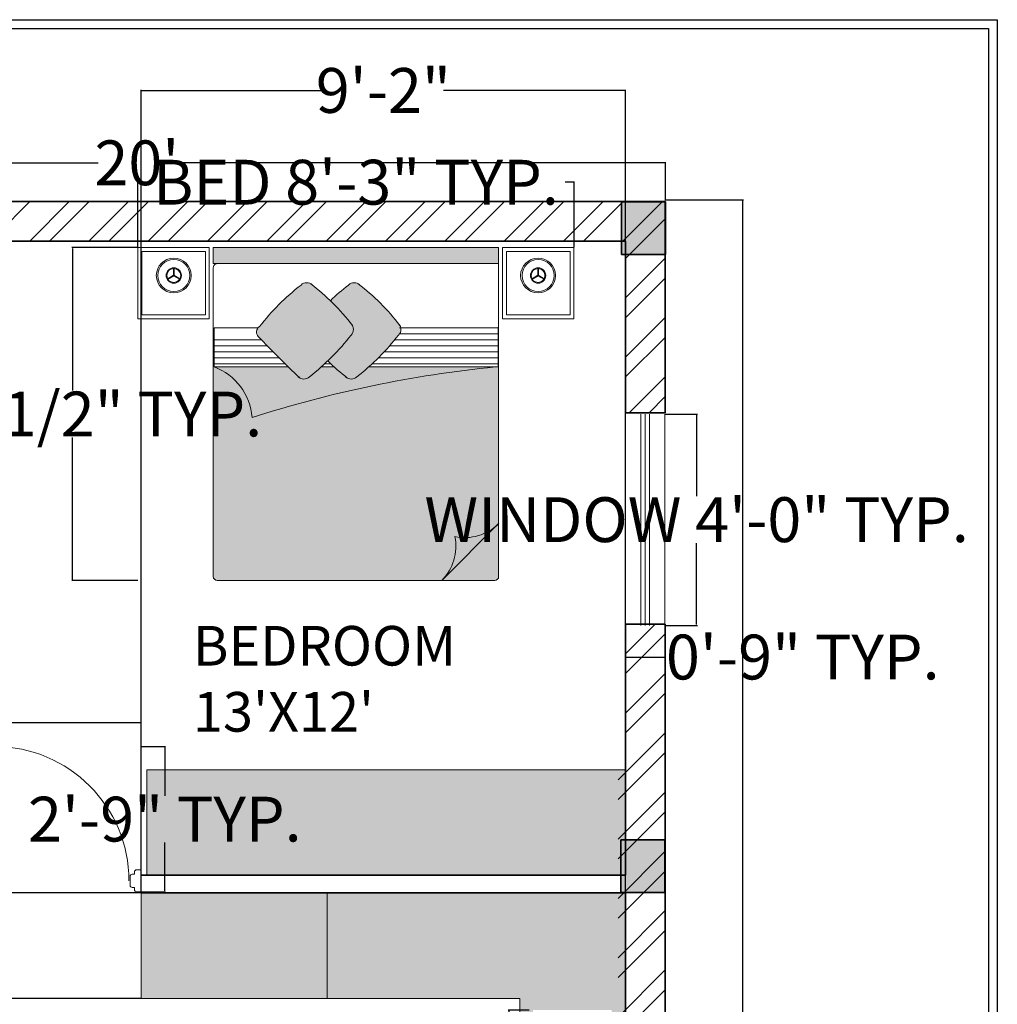
# Model space of a CAD drawing. Units: inches. Extents: x 1812 to 2791, y 2306 to 2959.
# Tile 4 of 8: x 1984 to 2206, y 2715 to 2939. Entities that reach past the tile are written whole.
import ezdxf

# ---------------------------------------------------------------- set-up
doc = ezdxf.new("R2010")
doc.units = ezdxf.units.IN
doc.layers.get('Defpoints').update_dxf_attribs({"lineweight": 50})
for name, color, linetype, lineweight in [('00 FURNITURE', 15, 'Continuous', 15), ('A-ANNO-DIMS', 2, 'Continuous', 18), ('A-ANNO-TTLB', 7, 'Continuous', 25), ('A-AREA-IDEN', 7, 'Continuous', 18), ('A-COLS', 7, 'Continuous', 35), ('A-FLOR-CASE', 8, 'Continuous', 18), ('A-WALL-PATT', 8, 'Continuous', 13), ('DOORS', 4, 'Continuous', 18), ('WALL', 7, 'Continuous', 35), ('WINDOWS', 160, 'Continuous', 18)]:
    doc.layers.add(name, color=color, linetype=linetype, lineweight=lineweight)
doc.layers.add('A-FURN-PATT', color=241, linetype='Continuous', lineweight=9, true_color=0xf7abae)
doc.styles.get("Standard").update_dxf_attribs({"font": 'arial.ttf'})
doc.dimstyles.get("Standard").update_dxf_attribs({"dimtxt": 10.18, "dimasz": 0.18, "dimexe": 0.18, "dimexo": 0.0625, "dimgap": 0.09, "dimtad": 0, "dimtih": 1, "dimtoh": 1, "dimdec": 0, "dimzin": 0, "dimdsep": 46, "dimlunit": 3, "dimtxsty": 'Standard', "dimcen": 0.09, "dimadec": 0, "dimazin": 0, "dimtfac": 1, "dimtdec": 0, "dimtofl": 0, "dimtmove": 0, "dimatfit": 3, "dimfxl": 1, "dimtolj": 1, "dimtzin": 0, "dimarcsym": 0})

# ---------------------------------------------------------------- blocks, each defined once
blk = doc.blocks.new('RGWTG')
at = {"layer": '00 FURNITURE'}
for p, q in [((578.23, 3473.51), (577.36, 3475.01)), ((578.23, 3473.58), (577.36, 3472.08)), ((578.36, 3473.58), (577.49, 3475.09)), ((578.36, 3473.51), (577.49, 3472)), ((578.29, 3473.62), (580.03, 3473.62)), ((578.29, 3473.47), (580.03, 3473.47)), ((521.93, 3464.58), (509.03, 3451.68)), ((509.93, 3464.58), (566.4, 3464.58)), ((557.53, 3463.84), (557.53, 3464.49)), ((557.53, 3464.49), (566.4, 3464.49)), ((558.2, 3464.49), (558.2, 3435.82)), ((559.57, 3464.49), (559.57, 3437.25)), ((560.94, 3464.49), (560.94, 3438.58)), ((562.3, 3464.49), (562.3, 3439.83)), ((563.67, 3464.49), (563.67, 3440.99)), ((565.04, 3464.49), (565.04, 3442.08)), ((566.4, 3464.58), (580.98, 3464.58)), ((566.4, 3464.49), (566.4, 3442.08)), ((566.4, 3464.49), (566.4, 3463.84)), ((580.98, 3464.58), (580.98, 3416.72)), ((509.03, 3422.63), (509.03, 3463.68)), ((558.2, 3426.48), (558.2, 3425.04)), ((509.03, 3400.68), (509.03, 3422.63)), ((558.2, 3416.13), (558.2, 3399.95)), ((580.98, 3416.72), (580.98, 3400.68)), ((559.57, 3414.75), (559.57, 3399.95)), ((560.94, 3413.39), (560.94, 3399.95)), ((562.3, 3412.04), (562.3, 3399.95)), ((563.67, 3410.72), (563.67, 3399.95)), ((580.08, 3399.78), (509.93, 3399.78)), ((557.53, 3399.95), (557.53, 3400.6)), ((566.4, 3399.95), (557.53, 3399.95)), ((566.4, 3400.6), (566.4, 3399.95)), ((578.23, 3390.78), (577.36, 3392.29)), ((578.23, 3390.86), (577.36, 3389.36)), ((578.36, 3390.86), (577.49, 3392.36)), ((578.36, 3390.78), (577.49, 3389.28)), ((578.29, 3390.9), (580.03, 3390.9)), ((578.29, 3390.74), (580.03, 3390.74))]:
    blk.add_line(p, q, dxfattribs=at)
for points in [[(568.43, 3465.48), (584.63, 3465.48), (584.63, 3481.68), (568.43, 3481.68)], [(569.33, 3466.38), (583.73, 3466.38), (583.73, 3480.78), (569.33, 3480.78)], [(580.98, 3399.78), (584.63, 3399.78), (584.63, 3464.58), (580.98, 3464.58)], [(568.43, 3398.88), (584.63, 3398.88), (584.63, 3382.68), (568.43, 3382.68)], [(569.33, 3397.98), (583.73, 3397.98), (583.73, 3383.58), (569.33, 3383.58)]]:
    blk.add_lwpolyline(points, close=True, dxfattribs=at)
for points in [[(566.52, 3464.49), (557.53, 3464.49), (557.53, 3435.08)], [(557.53, 3427.21), (557.53, 3424.3)], [(557.53, 3416.82), (557.53, 3399.95), (566.4, 3399.95), (566.4, 3409.94)]]:
    blk.add_lwpolyline(points, dxfattribs=at)
for centre, radius in [((578.29, 3473.54), 3.97), ((578.29, 3473.54), 3.63), ((578.29, 3473.54), 1.74), ((578.29, 3473.54), 1.56), ((578.29, 3390.82), 3.97), ((578.29, 3390.82), 3.63), ((578.29, 3390.82), 1.74), ((578.29, 3390.82), 1.56)]:
    blk.add_circle(centre, radius, dxfattribs=at)
for centre, radius, start, end in [((509.93, 3463.68), 0.9, 90, 180), ((529.65, 3456.88), 10.9, 135.0361, 191.9278), ((290.56, 3490.52), 268.3, 342.2214, 354.2925), ((516.73, 3443.97), 10.9, 78.0722, 134.9639), ((566.05, 3440.57), 1.82, 45, 135), ((533.58, 3399.31), 54.32, 37.931, 52.069), ((598.15, 3399.01), 54.32, 127.931, 142.069), ((574.84, 3431.77), 1.82, 315, 45), ((556.59, 3431.11), 1.82, 135, 225), ((598.15, 3388.23), 54.32, 127.931, 142.069), ((566.05, 3429.78), 1.82, 45, 135), ((533.58, 3388.53), 54.32, 37.931, 52.069), ((597.87, 3463.6), 54.32, 217.931, 224.141), ((533.28, 3463.88), 54.32, 316.32, 322.069), ((574.84, 3420.99), 1.82, 315, 45), ((556.59, 3420.33), 1.82, 135, 225), ((533.28, 3453.1), 54.32, 307.931, 322.069), ((765.33, 3619.75), 290.45, 223.6069, 226.2326), ((545.02, 3395.29), 13.35, 20.4224, 85.5825), ((565.44, 3411.05), 1.47, 225.9674, 326.8337), ((509.93, 3400.68), 0.9, 180, 270), ((580.08, 3400.68), 0.9, 270, 0)]:
    blk.add_arc(centre, radius, start, end, dxfattribs=at)
blk = doc.blocks.new('DDD')
at = {"layer": '00 FURNITURE'}
for p, q in [((-12579.77, -15859.53), (-12579.77, -15829.05)), ((-12578.77, -15859.53), (-12578.77, -15829.03)), ((-12612.02, -15857.03), (-12612.02, -15862.03)), ((-12611.02, -15857.03), (-12612.02, -15857.03)), ((-12610.52, -15858.03), (-12610.52, -15857.53)), ((-12577.52, -15858.03), (-12577.52, -15857.53)), ((-12577.02, -15857.03), (-12576.02, -15857.03)), ((-12576.02, -15857.03), (-12576.02, -15862.03)), ((-12578.77, -15859.53), (-12579.77, -15859.53)), ((-12612.02, -15862.03), (-12611.02, -15862.03)), ((-12610.52, -15861.53), (-12610.52, -15861.03)), ((-12577.52, -15861.53), (-12577.52, -15861.03)), ((-12576.02, -15862.03), (-12577.02, -15862.03))]:
    blk.add_line(p, q, dxfattribs=at)
for points in [[(-12610.52, -15861.03), (-12610.02, -15861.03, 0.414214), (-12609.52, -15860.53), (-12609.52, -15858.53, 0.414214), (-12610.02, -15858.03), (-12610.52, -15858.03)], [(-12577.52, -15861.03), (-12578.02, -15861.03, -0.414214), (-12578.52, -15860.53), (-12578.52, -15858.53, -0.414214), (-12578.02, -15858.03), (-12577.52, -15858.03)]]:
    blk.add_lwpolyline(points, format="xyb", dxfattribs=at)
for centre, radius, start, end in [((-12578.77, -15859.53), 30.5, 90, 180), ((-12611.02, -15857.53), 0.5, 0, 90), ((-12577.02, -15857.53), 0.5, 90, 180), ((-12611.02, -15861.53), 0.5, 270, 0), ((-12577.02, -15861.53), 0.5, 180, 270)]:
    blk.add_arc(centre, radius, start, end, dxfattribs=at)
blk = doc.blocks.new('*D14')
at = {"layer": 'A-ANNO-DIMS', "color": 0, "lineweight": -2, "transparency": 16777216}
for p, q in [((1890.37, 2897.89), (1890.37, 2906.59)), ((1890.55, 2906.41), (2001.61, 2906.41)), ((2130.3, 2906.41), (2019.24, 2906.41)), ((2130.48, 2897.89), (2130.48, 2906.59))]:
    blk.add_line(p, q, dxfattribs=at)
at = {"layer": 'A-ANNO-DIMS', "color": 0, "transparency": 16777216}
for points in [[(1890.55, 2906.44), (1890.55, 2906.38), (1890.37, 2906.41)], [(2130.3, 2906.44), (2130.3, 2906.38), (2130.48, 2906.41)]]:
    blk.add_solid(points, dxfattribs=at)
at = {"layer": 'Defpoints', "color": 0, "transparency": 16777216}
for p in [(2130.48, 2906.41), (1890.37, 2897.82), (2130.48, 2897.82)]:
    blk.add_point(p, dxfattribs=at)
at = {"layer": 'A-ANNO-DIMS', "color": 0, "transparency": 16777216, "insert": (2010.42, 2906.41), "char_height": 10.18, "attachment_point": 5}
blk.add_mtext("\\A1;20'", dxfattribs=at)
blk = doc.blocks.new('*D15')
at = {"layer": 'A-ANNO-DIMS', "color": 0, "lineweight": -2, "transparency": 16777216}
for p, q in [((2130.4, 2898), (2148.13, 2898)), ((2147.95, 2897.82), (2147.95, 2663.08)), ((2147.95, 2417.77), (2147.95, 2652.51)), ((2130.4, 2417.59), (2148.13, 2417.59))]:
    blk.add_line(p, q, dxfattribs=at)
at = {"layer": 'A-ANNO-DIMS', "color": 0, "transparency": 16777216}
for points in [[(2147.92, 2897.82), (2147.98, 2897.82), (2147.95, 2898)], [(2147.92, 2417.77), (2147.98, 2417.77), (2147.95, 2417.59)]]:
    blk.add_solid(points, dxfattribs=at)
at = {"layer": 'Defpoints', "color": 0, "transparency": 16777216}
for p in [(2130.34, 2898), (2130.34, 2417.59), (2147.95, 2417.59)]:
    blk.add_point(p, dxfattribs=at)
at = {"layer": 'A-ANNO-DIMS', "color": 0, "transparency": 16777216, "insert": (2147.95, 2657.8), "char_height": 10.18, "attachment_point": 5}
blk.add_mtext("\\A1;40'", dxfattribs=at)
blk = doc.blocks.new('COL')
at = {"transparency": 33554687}
h = blk.add_hatch(color=256, dxfattribs=at)
h.dxf.hatch_style = 1
h.paths.add_polyline_path([(2424.4, 2829.24), (2424.4, 2839.24), (2412.4, 2839.24), (2412.4, 2829.24)])
for p, q in [((2412.4, 2839.24), (2424.4, 2839.24)), ((2412.4, 2839.24), (2412.4, 2829.24)), ((2424.4, 2839.24), (2424.4, 2829.24)), ((2412.4, 2829.24), (2424.4, 2829.24))]:
    blk.add_line(p, q)
blk = doc.blocks.new('WINDOW-48x9')
for p, q in [((0, 48), (0, 0)), ((3.5, 0), (3.5, 48)), ((4.5, 0), (4.5, 48)), ((5.5, 0), (5.5, 48)), ((9, 0), (9, 48))]:
    blk.add_line(p, q)
blk = doc.blocks.new('SHEET-FRAME-RESIDENCE')
blk.add_lwpolyline([(0, 632.8), (378.76, 632.8), (378.76, 0), (0, 0)], close=True)
blk.add_lwpolyline([(2, 71.32), (2, 630.8), (376.76, 630.8), (376.76, 71.32)])
blk = doc.blocks.new('*D42')
at = {"layer": 'A-ANNO-DIMS', "color": 0, "lineweight": -2, "transparency": 16777216}
for p, q in [((1975.37, 2779.24), (1975.19, 2779.24)), ((1975.37, 2773.9), (1975.37, 2779.42)), ((2011.19, 2779.24), (1975.55, 2779.24)), ((2011.37, 2773.9), (2011.37, 2779.42))]:
    blk.add_line(p, q, dxfattribs=at)
at = {"layer": 'A-ANNO-DIMS', "color": 0, "transparency": 16777216}
for points in [[(1975.55, 2779.27), (1975.55, 2779.21), (1975.37, 2779.24)], [(2011.19, 2779.27), (2011.19, 2779.21), (2011.37, 2779.24)]]:
    blk.add_solid(points, dxfattribs=at)
at = {"layer": 'Defpoints', "color": 0, "transparency": 16777216}
for p in [(1975.37, 2779.24), (1975.37, 2773.84), (2011.37, 2773.84)]:
    blk.add_point(p, dxfattribs=at)
at = {"layer": 'A-ANNO-DIMS', "color": 0, "transparency": 16777216, "insert": (1921.02, 2779.24), "char_height": 10.18, "attachment_point": 5}
blk.add_mtext('\\A1;DOOR 3\'-0" TYP.', dxfattribs=at)
blk = doc.blocks.new('*D43')
at = {"layer": 'A-ANNO-DIMS', "color": 0, "lineweight": -2, "transparency": 16777216}
for p, q in [((2011.43, 2773.84), (2016.95, 2773.84)), ((2016.77, 2773.66), (2016.77, 2762.62)), ((2016.77, 2741.02), (2016.77, 2752.05)), ((2011.43, 2740.84), (2016.95, 2740.84))]:
    blk.add_line(p, q, dxfattribs=at)
at = {"layer": 'A-ANNO-DIMS', "color": 0, "transparency": 16777216}
for points in [[(2016.74, 2773.66), (2016.8, 2773.66), (2016.77, 2773.84)], [(2016.74, 2741.02), (2016.8, 2741.02), (2016.77, 2740.84)]]:
    blk.add_solid(points, dxfattribs=at)
at = {"layer": 'Defpoints', "color": 0, "transparency": 16777216}
for p in [(2011.37, 2773.84), (2016.77, 2773.84), (2011.37, 2740.84)]:
    blk.add_point(p, dxfattribs=at)
at = {"layer": 'A-ANNO-DIMS', "color": 0, "transparency": 16777216, "insert": (2016.77, 2757.34), "char_height": 10.18, "attachment_point": 5}
blk.add_mtext('\\A1;2\'-9" TYP.', dxfattribs=at)
blk = doc.blocks.new('*D46')
at = {"layer": 'A-ANNO-DIMS', "color": 0, "lineweight": -2, "transparency": 16777216}
for p, q in [((2130.38, 2849.36), (2137.7, 2849.36)), ((2137.52, 2849.18), (2137.52, 2830.72)), ((2137.52, 2801.54), (2137.52, 2820.01)), ((2130.38, 2801.36), (2137.7, 2801.36))]:
    blk.add_line(p, q, dxfattribs=at)
at = {"layer": 'A-ANNO-DIMS', "color": 0, "transparency": 16777216}
for points in [[(2137.49, 2849.18), (2137.55, 2849.18), (2137.52, 2849.36)], [(2137.49, 2801.54), (2137.55, 2801.54), (2137.52, 2801.36)]]:
    blk.add_solid(points, dxfattribs=at)
at = {"layer": 'Defpoints', "color": 0, "transparency": 16777216}
for p in [(2130.32, 2849.36), (2137.52, 2849.36), (2130.32, 2801.36)]:
    blk.add_point(p, dxfattribs=at)
at = {"layer": 'A-ANNO-DIMS', "color": 0, "transparency": 16777216, "insert": (2137.52, 2825.36), "char_height": 10.18, "attachment_point": 5}
blk.add_mtext('\\A1;WINDOW 4\'-0" TYP.', dxfattribs=at)
blk = doc.blocks.new('*D47')
at = {"layer": 'A-ANNO-DIMS', "color": 0, "lineweight": -2, "transparency": 16777216}
for p, q in [((2121.32, 2801.3), (2121.32, 2793.98)), ((2130.32, 2801.3), (2130.32, 2793.98)), ((2121.5, 2794.16), (2130.14, 2794.16)), ((2130.32, 2794.16), (2130.5, 2794.16))]:
    blk.add_line(p, q, dxfattribs=at)
at = {"layer": 'A-ANNO-DIMS', "color": 0, "transparency": 16777216}
for points in [[(2121.5, 2794.19), (2121.5, 2794.13), (2121.32, 2794.16)], [(2130.14, 2794.19), (2130.14, 2794.13), (2130.32, 2794.16)]]:
    blk.add_solid(points, dxfattribs=at)
at = {"layer": 'Defpoints', "color": 0, "transparency": 16777216}
for p in [(2121.32, 2801.36), (2130.32, 2801.36), (2130.32, 2794.16)]:
    blk.add_point(p, dxfattribs=at)
at = {"layer": 'A-ANNO-DIMS', "color": 0, "transparency": 16777216, "insert": (2161.62, 2794.16), "char_height": 10.18, "attachment_point": 5}
blk.add_mtext('\\A1;0\'-9" TYP.', dxfattribs=at)
blk = doc.blocks.new('*D50')
at = {"layer": 'A-ANNO-DIMS', "color": 0, "lineweight": -2, "transparency": 16777216}
for p, q in [((2010.68, 2887.22), (2010.68, 2902.19)), ((2010.86, 2902.01), (2012.69, 2902.01)), ((2109.5, 2902.01), (2107.66, 2902.01)), ((2109.68, 2887.22), (2109.68, 2902.19))]:
    blk.add_line(p, q, dxfattribs=at)
at = {"layer": 'A-ANNO-DIMS', "color": 0, "transparency": 16777216}
for points in [[(2010.86, 2902.04), (2010.86, 2901.98), (2010.68, 2902.01)], [(2109.5, 2902.04), (2109.5, 2901.98), (2109.68, 2902.01)]]:
    blk.add_solid(points, dxfattribs=at)
at = {"layer": 'Defpoints', "color": 0, "transparency": 16777216}
for p in [(2109.68, 2902.01), (2010.68, 2887.16), (2109.68, 2887.16)]:
    blk.add_point(p, dxfattribs=at)
at = {"layer": 'A-ANNO-DIMS', "color": 0, "transparency": 16777216, "insert": (2060.18, 2902.01), "char_height": 10.18, "attachment_point": 5}
blk.add_mtext('\\A1;BED 8\'-3" TYP.', dxfattribs=at)
blk = doc.blocks.new('*D51')
at = {"layer": 'A-ANNO-DIMS', "color": 0, "lineweight": -2, "transparency": 16777216}
for p, q in [((2010.61, 2887.16), (1995.65, 2887.16)), ((1995.83, 2886.98), (1995.83, 2854.71)), ((1995.83, 2811.74), (1995.83, 2844)), ((2010.61, 2811.56), (1995.65, 2811.56))]:
    blk.add_line(p, q, dxfattribs=at)
at = {"layer": 'A-ANNO-DIMS', "color": 0, "transparency": 16777216}
for points in [[(1995.8, 2886.98), (1995.86, 2886.98), (1995.83, 2887.16)], [(1995.8, 2811.74), (1995.86, 2811.74), (1995.83, 2811.56)]]:
    blk.add_solid(points, dxfattribs=at)
at = {"layer": 'Defpoints', "color": 0, "transparency": 16777216}
for p in [(1995.83, 2887.16), (2010.68, 2887.16), (2010.68, 2811.56)]:
    blk.add_point(p, dxfattribs=at)
at = {"layer": 'A-ANNO-DIMS', "color": 0, "transparency": 16777216, "insert": (1995.83, 2849.36), "char_height": 10.18, "attachment_point": 5}
blk.add_mtext('\\A1;6\'-3 1/2" TYP.', dxfattribs=at)
blk = doc.blocks.new('*D62')
at = {"layer": 'A-ANNO-DIMS', "color": 0, "lineweight": -2, "transparency": 16777216}
for p, q in [((2099.52, 2713.96), (2094.73, 2713.96)), ((2094.91, 2713.78), (2094.91, 2703.76)), ((2094.91, 2683.03), (2094.91, 2693.05)), ((2099.52, 2682.85), (2094.73, 2682.85))]:
    blk.add_line(p, q, dxfattribs=at)
at = {"layer": 'A-ANNO-DIMS', "color": 0, "transparency": 16777216}
for points in [[(2094.88, 2713.78), (2094.94, 2713.78), (2094.91, 2713.96)], [(2094.88, 2683.03), (2094.94, 2683.03), (2094.91, 2682.85)]]:
    blk.add_solid(points, dxfattribs=at)
at = {"layer": 'Defpoints', "color": 0, "transparency": 16777216}
for p in [(2094.91, 2713.96), (2099.58, 2713.96), (2099.58, 2682.85)]:
    blk.add_point(p, dxfattribs=at)
at = {"layer": 'A-ANNO-DIMS', "color": 0, "transparency": 16777216, "insert": (2094.91, 2698.41), "char_height": 10.18, "attachment_point": 5}
blk.add_mtext('\\A1;HOB 2\'-7" TYP.', dxfattribs=at)
blk = doc.blocks.new('*D81')
at = {"layer": 'A-ANNO-DIMS', "color": 0, "lineweight": -2, "transparency": 16777216}
for p, q in [((2011.32, 2740.6), (1864.78, 2740.6)), ((1864.96, 2740.42), (1864.96, 2733.89)), ((1864.96, 2716.78), (1864.96, 2723.32)), ((2011.32, 2716.6), (1864.78, 2716.6))]:
    blk.add_line(p, q, dxfattribs=at)
at = {"layer": 'A-ANNO-DIMS', "color": 0, "transparency": 16777216}
for points in [[(1864.93, 2740.42), (1864.99, 2740.42), (1864.96, 2740.6)], [(1864.93, 2716.78), (1864.99, 2716.78), (1864.96, 2716.6)]]:
    blk.add_solid(points, dxfattribs=at)
at = {"layer": 'Defpoints', "color": 0, "transparency": 16777216}
for p in [(2011.39, 2740.6), (1864.96, 2716.6), (2011.39, 2716.6)]:
    blk.add_point(p, dxfattribs=at)
at = {"layer": 'A-ANNO-DIMS', "color": 0, "transparency": 16777216, "insert": (1864.96, 2728.6), "char_height": 10.18, "attachment_point": 5}
blk.add_mtext('\\A1;2\'-0"', dxfattribs=at)
blk = doc.blocks.new('*D83')
at = {"layer": 'A-ANNO-DIMS', "color": 0, "lineweight": -2, "transparency": 16777216}
for p, q in [((2011.39, 2740.67), (2011.39, 2923.03)), ((2121.39, 2740.67), (2121.39, 2923.03)), ((2011.57, 2922.85), (2052.77, 2922.85)), ((2121.21, 2922.85), (2080.01, 2922.85))]:
    blk.add_line(p, q, dxfattribs=at)
at = {"layer": 'A-ANNO-DIMS', "color": 0, "transparency": 16777216}
for points in [[(2011.57, 2922.88), (2011.57, 2922.82), (2011.39, 2922.85)], [(2121.21, 2922.88), (2121.21, 2922.82), (2121.39, 2922.85)]]:
    blk.add_solid(points, dxfattribs=at)
at = {"layer": 'Defpoints', "color": 0, "transparency": 16777216}
for p in [(2121.39, 2922.85), (2011.39, 2740.6), (2121.39, 2740.6)]:
    blk.add_point(p, dxfattribs=at)
at = {"layer": 'A-ANNO-DIMS', "color": 0, "transparency": 16777216, "insert": (2066.39, 2922.85), "char_height": 10.18, "attachment_point": 5}
blk.add_mtext('\\A1;9\'-2"', dxfattribs=at)

msp = doc.modelspace()

# ---------------------------------------------------------------- hatches: boundary and pattern name
at = {"layer": 'A-FURN-PATT', "transparency": 33554534}
h = msp.add_hatch(color=256, dxfattribs=at)
h.dxf.hatch_style = 1
h.paths.add_polyline_path([(2121.39, 2740.6), (2053.61, 2740.6), (2053.61, 2716.6), (2097.39, 2716.6), (2097.39, 2656.6), (2059.39, 2656.6), (2059.39, 2632.6), (2067.87, 2632.6), (2067.87, 2631.77), (2115.87, 2631.77), (2115.87, 2632.6), (2121.39, 2632.6)])
h.paths.add_polyline_path([(2100.36, 2713.96), (2118.26, 2713.96), (2118.26, 2682.85), (2100.36, 2682.85), (2100.36, 2684.81), (2099.58, 2684.81), (2099.58, 2711.69), (2100.36, 2711.69)], flags=16)
h.paths.add_polyline_path([(2111.2, 2707.14, -1), (2104.93, 2707.14, -1)], flags=0)
h.paths.add_polyline_path([(2111.59, 2690.39, -1), (2104.53, 2690.39, -1)], flags=0)
h.paths.add_polyline_path([(2121.35, 2768.56), (2012.67, 2768.56), (2012.67, 2744.6), (2121.35, 2744.6)])
h.paths.add_polyline_path([(2053.61, 2740.6), (2011.39, 2740.6), (2011.39, 2716.6), (2053.61, 2716.6)])
h.paths.add_polyline_path([(1935.43, 2537.08), (1909.15, 2537.08), (1909.15, 2510.8), (1935.43, 2510.8)])
h.paths.add_polyline_path([(1935.43, 2560.67, 0.414214), (1933.24, 2562.86), (1909.15, 2562.86), (1909.15, 2537.08), (1935.43, 2537.08)])
h.paths.add_polyline_path([(1966.09, 2581.45), (1939.81, 2581.45), (1939.81, 2557.36, 0.414214), (1942, 2555.17), (1963.9, 2555.17, 0.414214), (1966.09, 2557.36)])
h.paths.add_polyline_path([(1935.43, 2510.8), (1909.15, 2510.8), (1909.15, 2485.01), (1933.24, 2485.01, 0.414214), (1935.43, 2487.2)])
h.paths.add_polyline_path([(1967.42, 2494.07, 0.414214), (1965.23, 2496.26), (1943.33, 2496.26, 0.414214), (1941.14, 2494.07), (1941.14, 2469.98), (1967.42, 2469.98)])
h.paths.add_polyline_path([(2050.11, 2878.8, 0.308459), (2048.07, 2878.94, 0.065472), (2038.04, 2868.93), (2037.94, 2868.93, 0.386143), (2037.98, 2866.96, 0.011497), (2047.44, 2857.53, 0.265248), (2049.25, 2857.55, 0.066056), (2059.35, 2867.65, 0.308904), (2059.21, 2869.7, 0.059418)])
h.paths.add_polyline_path([(2060.9, 2878.8, 0.308459), (2058.85, 2878.94, 0.027227), (2054.36, 2875.09, -0.033416), (2059.21, 2869.71, -0.379362), (2059.07, 2867.29, -0.036525), (2053.76, 2861.41, 0.027343), (2058.24, 2857.52, 0.262295), (2060.03, 2857.55, 0.066056), (2070.13, 2867.65, 0.308904), (2070, 2869.7, 0.059418)])
h.paths.add_polyline_path([(2092.58, 2824.46), (2079.67, 2811.56), (2091.68, 2811.56, 0.414214), (2092.58, 2812.46)], flags=17)
h.paths.add_polyline_path([(2092.58, 2860.06), (2091.83, 2860.06, 0.052719), (2036.59, 2848.58, 0.295777), (2027.78, 2860.12), (2027.78, 2812.46, 0.414214), (2028.68, 2811.56), (2050.63, 2811.56), (2079.67, 2811.56, 0.253465), (2082.62, 2821.51, 0.253465), (2092.58, 2824.46)])
h.paths.add_polyline_path([(2091.83, 2860.06), (2063.07, 2860.06, -0.016036), (2060.39, 2857.83, -0.429576), (2057.75, 2857.9, -0.015371), (2055.2, 2860.06), (2052.29, 2860.06, -0.016036), (2049.61, 2857.83, -0.334836), (2047.44, 2857.53, -0.003141), (2044.81, 2860.06), (2027.94, 2860.06, -0.292232), (2036.59, 2848.58, -0.052719)], flags=17)
h.paths.add_polyline_path([(2092.59, 2824.47, -0.2538), (2082.62, 2821.51, -0.253465), (2079.67, 2811.56)])
h.paths.add_polyline_path([(2092.58, 2887.16), (2027.78, 2887.16), (2027.78, 2883.51), (2092.58, 2883.51)])
at = {"layer": 'A-WALL-PATT'}
h = msp.add_hatch(dxfattribs=at)
h.set_pattern_fill('ANSI32', color=256)
h.paths.add_polyline_path([(2130.39, 2417.6), (2119.69, 2417.6), (2119.69, 2768.56), (2121.39, 2768.56), (2121.39, 2801.62), (2121.32, 2849.36), (2121.32, 2801.62), (2130.39, 2801.62)])
h.paths.add_polyline_path([(2023.39, 2426.6), (1899.39, 2426.6), (1899.39, 2453.6), (1951.8, 2453.6), (1951.8, 2457.6), (1899.39, 2457.6), (1899.39, 2590.6), (1959.93, 2590.6), (1959.93, 2594.6), (1899.39, 2594.6), (1899.39, 2634.53), (1890.39, 2634.53), (1890.39, 2417.6), (2023.39, 2417.6)])
h.paths.add_polyline_path([(2119.69, 2426.6), (2112.39, 2426.6), (2112.39, 2417.6), (2119.69, 2417.6)])
h.paths.add_polyline_path([(1899.39, 2740.6), (1941.39, 2740.6), (1941.39, 2744.6), (1899.39, 2744.6), (1899.39, 2772.94), (1890.39, 2772.94), (1890.39, 2682.53), (1899.21, 2682.53), (1899.21, 2682.64)])
h.paths.add_polyline_path([(1975.39, 2838.6), (1899.39, 2838.6), (1899.39, 2856.33), (1890.39, 2856.33), (1890.39, 2796.95), (1899.39, 2796.95), (1899.39, 2834.6), (1971.39, 2834.6), (1971.39, 2740.6), (1975.39, 2740.6)])
h.paths.add_polyline_path([(2119.69, 2897.6), (1890.39, 2897.6), (1890.39, 2880.36), (1899.39, 2880.36), (1899.39, 2888.6), (2119.69, 2888.6)])
h.paths.add_polyline_path([(2130.39, 2897.6), (2119.69, 2897.6), (2119.69, 2888.6), (2121.39, 2888.6), (2121.39, 2849.62), (2130.39, 2849.62)])

# ---------------------------------------------------------------- linework, layer by layer
at = {"layer": 'A-FLOR-CASE'}
for p, q in [((2121.35, 2768.56), (2012.67, 2768.56)), ((2012.67, 2744.6), (2012.67, 2768.56)), ((2121.35, 2744.56), (2121.35, 2768.56)), ((2011.39, 2716.6), (2011.39, 2744.6)), ((2053.61, 2716.6), (2053.61, 2740.6)), ((2011.39, 2716.6), (2097.39, 2716.6)), ((2097.39, 2716.6), (2097.39, 2656.6))]:
    msp.add_line(p, q, dxfattribs=at)
at = {"layer": 'WALL'}
for p, q in [((1890.39, 2897.6), (2130.39, 2897.6)), ((2130.39, 2897.6), (2130.39, 2849.62)), ((1899.39, 2888.6), (2121.39, 2888.6)), ((2121.39, 2888.6), (2121.39, 2849.62)), ((2121.39, 2849.62), (2130.39, 2849.62)), ((2121.39, 2801.62), (2121.39, 2744.6)), ((2121.39, 2801.62), (2130.39, 2801.62)), ((2121.39, 2801.62), (2121.39, 2744.6)), ((2130.39, 2801.62), (2130.39, 2417.6)), ((2011.39, 2744.6), (2121.39, 2744.6)), ((2011.39, 2740.6), (2055.39, 2740.6)), ((2011.39, 2740.6), (2121.39, 2740.6)), ((2121.39, 2740.6), (2121.39, 2632.6))]:
    msp.add_line(p, q, dxfattribs=at)

# ---------------------------------------------------------------- block references
at = {"layer": '00 FURNITURE', "xscale": -1, "rotation": 270}
msp.add_blockref('RGWTG', (-1372.01, 2302.53), dxfattribs=at)
at = {"layer": 'A-ANNO-TTLB'}
msp.add_blockref('SHEET-FRAME-RESIDENCE', (1827.03, 2306.12), dxfattribs=at)
at = {"layer": 'A-COLS', "rotation": 270}
for p in [(-708.79, 5309.97), (-708.95, 5165.04)]:
    msp.add_blockref('COL', p, dxfattribs=at)
at = {"layer": 'DOORS', "xscale": -1}
msp.add_blockref('DDD', (-10600.65, 18602.87), dxfattribs=at)
at = {"layer": 'WINDOWS'}
msp.add_blockref('WINDOW-48x9', (2121.32, 2801.36), dxfattribs=at)

# ---------------------------------------------------------------- texts
at = {"layer": 'A-AREA-IDEN', "insert": (2023.16, 2801.22), "char_height": 9, "attachment_point": 1}
msp.add_mtext_dynamic_manual_height_columns("BEDROOM\\P13'X12'", width=96.4869, gutter_width=12.5, heights=[0], dxfattribs=at)

# ---------------------------------------------------------------- dimensions: what is measured, and where the dimension line sits
at = {"layer": 'A-ANNO-DIMS'}
for base, p1, p2, override, picture, middle in [((2121.39, 2922.85), (2011.39, 2740.6), (2121.39, 2740.6), {"dimdec": 1, "dimlfac": 1, "dimrnd": 0, "dimzin": 1, "dimdsep": 46, "dimlunit": 4, "dimfrac": 2}, '*D83', (2066.39, 2922.85)), ((2130.48, 2906.41), (1890.37, 2897.82), (2130.48, 2897.82), {"dimclrd": 0, "dimclre": 0, "dimclrt": 0}, '*D14', (2010.42, 2906.41))]:
    dim = msp.add_linear_dim(base=base, p1=p1, p2=p2, dimstyle='Standard', override=override, dxfattribs=at)
    dim.commit()
    dim.dimension.update_dxf_attribs({"geometry": picture, "text_midpoint": middle})
for base, p1, p2, text, picture, middle in [((2109.68, 2902.01), (2010.68, 2887.16), (2109.68, 2887.16), 'BED <> TYP.', '*D50', (2060.18, 2902.01)), ((2130.32, 2794.16), (2121.32, 2801.36), (2130.32, 2801.36), '<> TYP.', '*D47', (2161.62, 2794.16))]:
    dim = msp.add_linear_dim(base=base, p1=p1, p2=p2, text=text, dimstyle='Standard', override={"dimdec": 1, "dimlfac": 1, "dimrnd": 0, "dimzin": 1, "dimdsep": 46, "dimlunit": 4, "dimfrac": 2}, dxfattribs=at)
    dim.commit()
    dim.dimension.update_dxf_attribs({"geometry": picture, "text_midpoint": middle})
dim = msp.add_linear_dim(base=(2147.95, 2417.59), p1=(2130.34, 2898), p2=(2130.34, 2417.59), angle=90, dimstyle='Standard', override={"dimclrd": 0, "dimclre": 0, "dimclrt": 0}, dxfattribs=at)
dim.commit()
dim.dimension.update_dxf_attribs({"geometry": '*D15', "text_midpoint": (2147.95, 2657.8), "dimtype": 160})
for base, p1, p2, angle, text, picture, middle in [((1995.83, 2887.16), (2010.68, 2811.56), (2010.68, 2887.16), 90, '<> TYP.', '*D51', (1995.83, 2849.36)), ((2137.52, 2849.36), (2130.32, 2801.36), (2130.32, 2849.36), 90, 'WINDOW <> TYP.', '*D46', (2137.52, 2825.36)), ((1975.37, 2779.24), (2011.37, 2773.84), (1975.37, 2773.84), 180, 'DOOR <> TYP.', '*D42', (1921.02, 2779.24)), ((2016.77, 2773.84), (2011.37, 2740.84), (2011.37, 2773.84), 90, '<> TYP.', '*D43', (2016.77, 2757.34)), ((2094.91, 2713.96), (2099.58, 2682.85), (2099.58, 2713.96), 90, 'HOB <> TYP.', '*D62', (2094.91, 2698.41))]:
    dim = msp.add_linear_dim(base=base, p1=p1, p2=p2, angle=angle, text=text, dimstyle='Standard', override={"dimdec": 1, "dimlfac": 1, "dimrnd": 0, "dimzin": 1, "dimdsep": 46, "dimlunit": 4, "dimfrac": 2}, dxfattribs=at)
    dim.commit()
    dim.dimension.update_dxf_attribs({"geometry": picture, "text_midpoint": middle})
dim = msp.add_linear_dim(base=(1864.96, 2716.6), p1=(2011.39, 2740.6), p2=(2011.39, 2716.6), angle=90, dimstyle='Standard', override={"dimdec": 1, "dimlfac": 1, "dimrnd": 0, "dimzin": 1, "dimdsep": 46, "dimlunit": 4, "dimfrac": 2}, dxfattribs=at)
dim.commit()
dim.dimension.update_dxf_attribs({"geometry": '*D81', "text_midpoint": (1864.96, 2728.6)})

doc.saveas('drawing.dxf')
